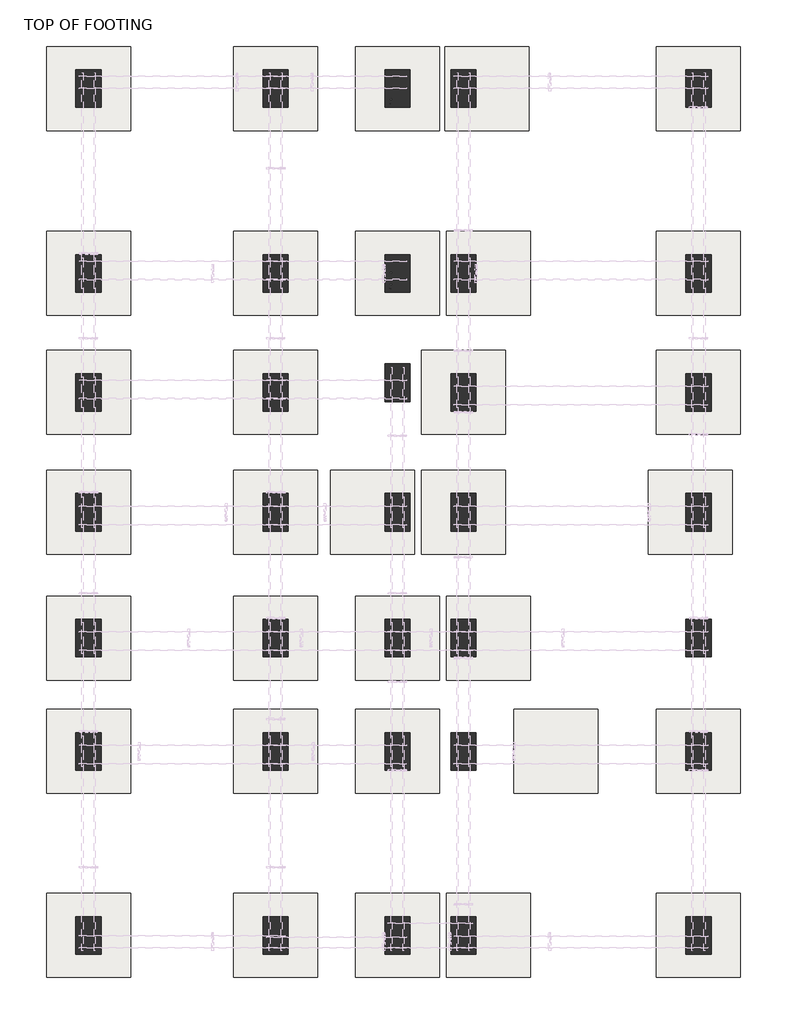
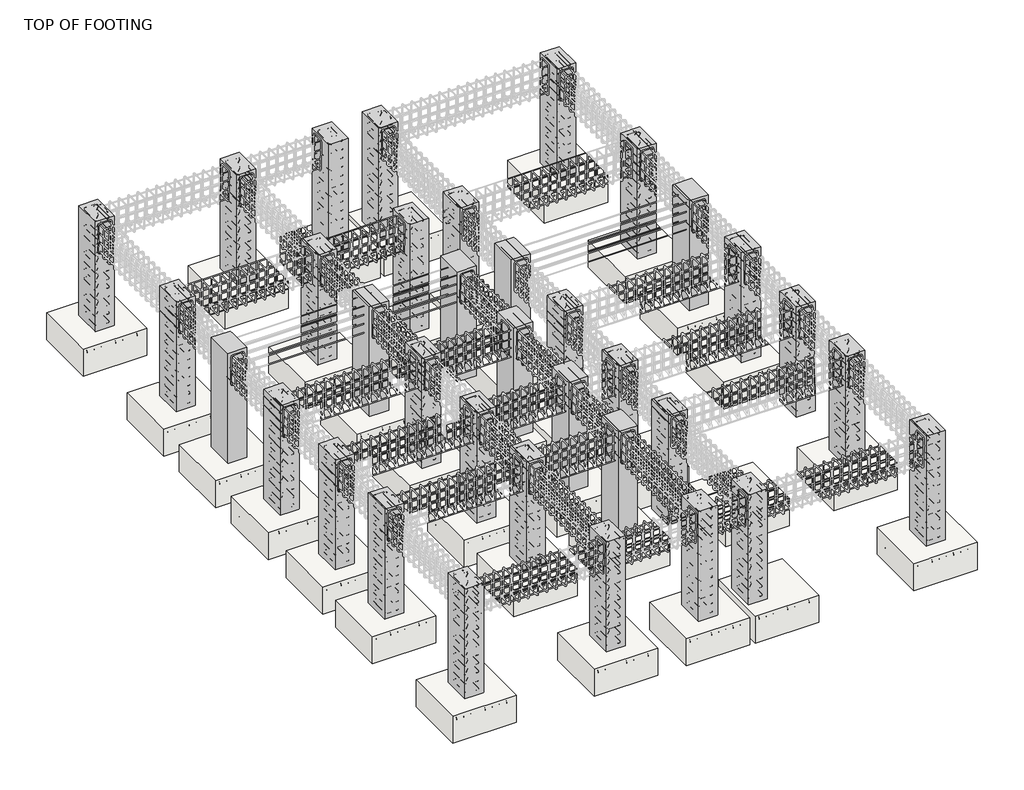
# One storey, part 1 of 19: 35 columns, 33 slabs.
"""IFC4 building model written with IfcOpenShell, lengths in millimetres."""

from ifc_helpers import new_model, si_unit, frame, origin, place, context, project, spatial, polyline, outline, extrude, faceted_brep, transform, mapped, element, save
from components import m_footing_rectangular_4c97ae35

model = new_model("IFC4")

# Units and contexts
model_context = context("Model", 3, world=origin())
ifc_project = project(units=[si_unit("LENGTHUNIT", "METRE", prefix="MILLI")], contexts=[model_context])

# Site, building, storey
site = spatial("IfcSite", under=ifc_project)
building = spatial("IfcBuilding", under=site)
storey = spatial("IfcBuildingStorey", under=building, Name="TOP OF FOOTING", Elevation=-1828.8)

# Columns
placement = place(None, origin())
element("IfcColumn", 1, ObjectType="M_Concrete-Rectangular-Column : 300 x 450mm", at=placement, inside=storey, context=model_context, shape_type="Brep", body=[
    faceted_brep([(-5487.6766954, 9387.4259714, -1828.8), (-5487.6766954, 8937.4259714, -1828.8), (-5787.6766954, 8937.4259714, -1828.8), (-5787.6766954, 9387.4259714, -1828.8), (-5487.6766954, 9387.4259714, 0.0), (-5487.6766954, 9087.4259714, 0.0), (-5487.6766954, 8937.4259714, 0.0), (-5787.6766954, 8937.4259714, 0.0), (-5787.6766954, 9387.4259714, 0.0)], [[[0, 1, 2, 3]], [[4, 5, 6, 1, 0]], [[6, 7, 2, 1]], [[7, 8, 3, 2]], [[8, 4, 0, 3]], [[4, 8, 7, 6, 5]]]),
])
element("IfcColumn", 2, ObjectType="M_Concrete-Rectangular-Column : 300 x 450mm", at=placement, inside=storey, context=model_context, shape_type="Brep", body=[
    faceted_brep([(-3258.2783472, 9387.4259714, -1828.8), (-3258.2783472, 8937.4259714, -1828.8), (-3558.2783472, 8937.4259714, -1828.8), (-3558.2783472, 9387.4259714, -1828.8), (-3258.2783472, 9387.4259714, 0.0), (-3258.2783472, 9087.4259714, 0.0), (-3258.2783472, 8937.4259714, 0.0), (-3558.2783472, 8937.4259714, 0.0), (-3558.2783472, 9087.4259714, 0.0), (-3558.2783472, 9387.4259714, 0.0)], [[[0, 1, 2, 3]], [[4, 5, 6, 1, 0]], [[6, 7, 2, 1]], [[7, 8, 9, 3, 2]], [[9, 4, 0, 3]], [[4, 9, 8, 7, 6, 5]]]),
])
element("IfcColumn", 3, ObjectType="M_Concrete-Rectangular-Column : 300 x 450mm", at=placement, inside=storey, context=model_context, shape_type="Brep", body=[
    faceted_brep([(-1807.6766954, 9387.4259714, -1828.8), (-1807.6766954, 8937.4259714, -1828.8), (-2107.6766954, 8937.4259714, -1828.8), (-2107.6766954, 9387.4259714, -1828.8), (-1807.6766954, 9387.4259714, 0.0), (-1807.6766954, 9087.4259714, 0.0), (-1807.6766954, 8937.4259714, 0.0), (-2107.6766954, 8937.4259714, 0.0), (-2107.6766954, 9087.4259714, 0.0), (-2107.6766954, 9387.4259714, 0.0)], [[[0, 1, 2, 3]], [[4, 5, 6, 1, 0]], [[6, 7, 2, 1]], [[7, 8, 9, 3, 2]], [[9, 4, 0, 3]], [[4, 9, 8, 7, 6, 5]]]),
])
element("IfcColumn", 4, ObjectType="M_Concrete-Rectangular-Column : 300 x 450mm", at=placement, inside=storey, context=model_context, shape_type="Brep", body=[
    faceted_brep([(-1022.4314918, 9387.4259714, -1828.8), (-1022.4314918, 8937.4259714, -1828.8), (-1322.4314918, 8937.4259714, -1828.8), (-1322.4314918, 9387.4259714, -1828.8), (-1022.4314918, 9387.4259714, 0.0), (-1022.4314918, 9087.4259714, 0.0), (-1022.4314918, 8937.4259714, 0.0), (-1322.4314918, 8937.4259714, 0.0), (-1322.4314918, 9087.4259714, 0.0), (-1322.4314918, 9387.4259714, 0.0)], [[[0, 1, 2, 3]], [[4, 5, 6, 1, 0]], [[6, 7, 2, 1]], [[7, 8, 9, 3, 2]], [[9, 4, 0, 3]], [[4, 9, 8, 7, 6, 5]]]),
])
element("IfcColumn", 5, ObjectType="M_Concrete-Rectangular-Column : 300 x 450mm", at=placement, inside=storey, context=model_context, shape_type="Brep", body=[
    faceted_brep([(1777.5685082, 9387.4259714, -1828.8), (1777.5685082, 8937.4259714, -1828.8), (1477.5685082, 8937.4259714, -1828.8), (1477.5685082, 9387.4259714, -1828.8), (1777.5685082, 9387.4259714, 0.0), (1777.5685082, 8937.4259714, 0.0), (1477.5685082, 8937.4259714, 0.0), (1477.5685082, 9087.4259714, 0.0), (1477.5685082, 9387.4259714, 0.0)], [[[0, 1, 2, 3]], [[4, 5, 1, 0]], [[5, 6, 2, 1]], [[6, 7, 8, 3, 2]], [[8, 4, 0, 3]], [[4, 8, 7, 6, 5]]]),
])
element("IfcColumn", 6, ObjectType="M_Concrete-Rectangular-Column : 300 x 450mm", at=placement, inside=storey, context=model_context, shape_type="Brep", body=[
    faceted_brep([(-5487.6766954, 7186.4301143, -1828.8), (-5487.6766954, 6736.4301143, -1828.8), (-5787.6766954, 6736.4301143, -1828.8), (-5787.6766954, 7186.4301143, -1828.8), (-5487.6766954, 7186.4301143, 0.0), (-5487.6766954, 7111.4301143, 0.0), (-5487.6766954, 6811.4301143, 0.0), (-5487.6766954, 6736.4301143, 0.0), (-5787.6766954, 6736.4301143, 0.0), (-5787.6766954, 7186.4301143, 0.0)], [[[0, 1, 2, 3]], [[4, 5, 6, 7, 1, 0]], [[7, 8, 2, 1]], [[8, 9, 3, 2]], [[9, 4, 0, 3]], [[4, 9, 8, 7, 6, 5]]]),
])
element("IfcColumn", 7, ObjectType="M_Concrete-Rectangular-Column : 300 x 450mm", at=placement, inside=storey, context=model_context, shape_type="Brep", body=[
    faceted_brep([(-3258.2783472, 7186.4301143, -1828.8), (-3258.2783472, 6736.4301143, -1828.8), (-3558.2783472, 6736.4301143, -1828.8), (-3558.2783472, 7186.4301143, -1828.8), (-3258.2783472, 7186.4301143, 0.0), (-3258.2783472, 7111.4301143, 0.0), (-3258.2783472, 6811.4301143, 0.0), (-3258.2783472, 6736.4301143, 0.0), (-3258.2783472, 6736.4301143, -300.0), (-3558.2783472, 6736.4301143, 0.0), (-3558.2783472, 6736.4301143, -300.0), (-3558.2783472, 6811.4301143, 0.0), (-3558.2783472, 7111.4301143, 0.0), (-3558.2783472, 7186.4301143, 0.0)], [[[0, 1, 2, 3]], [[1, 0, 4, 5, 6, 7, 8]], [[2, 1, 8, 7, 9, 10]], [[3, 2, 10, 9, 11, 12, 13]], [[0, 3, 13, 4]], [[9, 7, 6, 5, 4, 13, 12, 11]]]),
])
element("IfcColumn", 8, ObjectType="M_Concrete-Rectangular-Column : 300 x 450mm", at=placement, inside=storey, context=model_context, shape_type="Brep", body=[
    faceted_brep([(-1807.6766954, 7186.4301143, -1828.8), (-1807.6766954, 6736.4301143, -1828.8), (-2107.6766954, 6736.4301143, -1828.8), (-2107.6766954, 7186.4301143, -1828.8), (-1807.6766954, 7186.4301143, 0.0), (-1807.6766954, 7111.4301143, 0.0), (-1807.6766954, 6811.4301143, 0.0), (-1807.6766954, 6736.4301143, 0.0), (-1807.6766954, 6736.4301143, -300.0), (-2107.6766954, 6736.4301143, 0.0), (-2107.6766954, 6736.4301143, -300.0), (-2107.6766954, 6811.4301143, 0.0), (-2107.6766954, 7111.4301143, 0.0), (-2107.6766954, 7186.4301143, 0.0)], [[[0, 1, 2, 3]], [[1, 0, 4, 5, 6, 7, 8]], [[2, 1, 8, 7, 9, 10]], [[3, 2, 10, 9, 11, 12, 13]], [[0, 3, 13, 4]], [[9, 7, 6, 5, 4, 13, 12, 11]]]),
])
element("IfcColumn", 9, ObjectType="M_Concrete-Rectangular-Column : 300 x 450mm", at=placement, inside=storey, context=model_context, shape_type="Brep", body=[
    faceted_brep([(-1022.4314918, 7186.4301143, -1828.8), (-1022.4314918, 6736.4301143, -1828.8), (-1322.4314918, 6736.4301143, -1828.8), (-1322.4314918, 7186.4301143, -1828.8), (-1022.4314918, 7186.4301143, 0.0), (-1022.4314918, 7111.4301143, 0.0), (-1022.4314918, 6811.4301143, 0.0), (-1022.4314918, 6736.4301143, 0.0), (-1022.4314918, 6736.4301143, -300.0), (-1322.4314918, 6736.4301143, 0.0), (-1322.4314918, 6736.4301143, -300.0), (-1322.4314918, 6811.4301143, 0.0), (-1322.4314918, 7111.4301143, 0.0), (-1322.4314918, 7186.4301143, 0.0)], [[[0, 1, 2, 3]], [[1, 0, 4, 5, 6, 7, 8]], [[2, 1, 8, 7, 9, 10]], [[3, 2, 10, 9, 11, 12, 13]], [[0, 3, 13, 4]], [[9, 7, 6, 5, 4, 13, 12, 11]]]),
])
element("IfcColumn", 10, ObjectType="M_Concrete-Rectangular-Column : 300 x 450mm", at=placement, inside=storey, context=model_context, shape_type="Brep", body=[
    faceted_brep([(1777.5685082, 7186.4301143, -1828.8), (1777.5685082, 6736.4301143, -1828.8), (1477.5685082, 6736.4301143, -1828.8), (1477.5685082, 7186.4301143, -1828.8), (1777.5685082, 7186.4301143, 0.0), (1777.5685082, 6736.4301143, 0.0), (1477.5685082, 6736.4301143, 0.0), (1477.5685082, 6811.4301143, 0.0), (1477.5685082, 7111.4301143, 0.0), (1477.5685082, 7186.4301143, 0.0)], [[[0, 1, 2, 3]], [[4, 5, 1, 0]], [[5, 6, 2, 1]], [[6, 7, 8, 9, 3, 2]], [[9, 4, 0, 3]], [[4, 9, 8, 7, 6, 5]]]),
])
element("IfcColumn", 11, ObjectType="M_Concrete-Rectangular-Column : 300 x 450mm", at=placement, inside=storey, context=model_context, shape_type="Brep", body=[
    faceted_brep([(-5487.6766954, 5769.9548165, -1828.8), (-5487.6766954, 5319.9548165, -1828.8), (-5787.6766954, 5319.9548165, -1828.8), (-5787.6766954, 5769.9548165, -1828.8), (-5487.6766954, 5769.9548165, 0.0), (-5487.6766954, 5694.9548165, 0.0), (-5487.6766954, 5394.9548165, 0.0), (-5487.6766954, 5319.9548165, 0.0), (-5787.6766954, 5319.9548165, 0.0), (-5787.6766954, 5769.9548165, 0.0)], [[[0, 1, 2, 3]], [[4, 5, 6, 7, 1, 0]], [[7, 8, 2, 1]], [[8, 9, 3, 2]], [[9, 4, 0, 3]], [[4, 9, 8, 7, 6, 5]]]),
])
element("IfcColumn", 12, ObjectType="M_Concrete-Rectangular-Column : 300 x 450mm", at=placement, inside=storey, context=model_context, shape_type="Brep", body=[
    faceted_brep([(-3258.2783472, 5769.9548165, -1828.8), (-3258.2783472, 5319.9548165, -1828.8), (-3558.2783472, 5319.9548165, -1828.8), (-3558.2783472, 5769.9548165, -1828.8), (-3258.2783472, 5769.9548165, -300.0), (-3258.2783472, 5769.9548165, 0.0), (-3258.2783472, 5694.9548165, 0.0), (-3258.2783472, 5394.9548165, 0.0), (-3258.2783472, 5319.9548165, 0.0), (-3258.2783472, 5319.9548165, -300.0), (-3558.2783472, 5319.9548165, 0.0), (-3558.2783472, 5319.9548165, -300.0), (-3558.2783472, 5394.9548165, 0.0), (-3558.2783472, 5694.9548165, 0.0), (-3558.2783472, 5769.9548165, 0.0), (-3558.2783472, 5769.9548165, -300.0)], [[[0, 1, 2, 3]], [[1, 0, 4, 5, 6, 7, 8, 9]], [[2, 1, 9, 8, 10, 11]], [[3, 2, 11, 10, 12, 13, 14, 15]], [[0, 3, 15, 14, 5, 4]], [[10, 8, 7, 6, 5, 14, 13, 12]]]),
])
element("IfcColumn", 13, ObjectType="M_Concrete-Rectangular-Column : 300 x 450mm", at=placement, inside=storey, context=model_context, shape_type="Brep", body=[
    faceted_brep([(-1807.6766954, 5886.4301143, -1828.8), (-1807.6766954, 5436.4301143, -1828.8), (-2107.6766954, 5436.4301143, -1828.8), (-2107.6766954, 5886.4301143, -1828.8), (-1807.6766954, 5886.4301143, -300.0), (-1807.6766954, 5886.4301143, 0.0), (-1807.6766954, 5694.9548165, 0.0), (-1807.6766954, 5436.4301143, 0.0), (-2107.6766954, 5436.4301143, 0.0), (-2107.6766954, 5694.9548165, 0.0), (-2107.6766954, 5886.4301143, 0.0), (-2107.6766954, 5886.4301143, -300.0)], [[[0, 1, 2, 3]], [[1, 0, 4, 5, 6, 7]], [[2, 1, 7, 8]], [[3, 2, 8, 9, 10, 11]], [[0, 3, 11, 10, 5, 4]], [[8, 7, 6, 5, 10, 9]]]),
])
element("IfcColumn", 14, ObjectType="M_Concrete-Rectangular-Column : 300 x 450mm", at=placement, inside=storey, context=model_context, shape_type="Brep", body=[
    faceted_brep([(-1022.4314918, 5769.9548165, -1828.8), (-1022.4314918, 5319.9548165, -1828.8), (-1322.4314918, 5319.9548165, -1828.8), (-1322.4314918, 5769.9548165, -1828.8), (-1022.4314918, 5769.9548165, -300.0), (-1022.4314918, 5769.9548165, 0.0), (-1022.4314918, 5694.9548165, 0.0), (-1022.4314918, 5394.9548165, 0.0), (-1022.4314918, 5319.9548165, 0.0), (-1022.4314918, 5319.9548165, -300.0), (-1322.4314918, 5319.9548165, 0.0), (-1322.4314918, 5319.9548165, -300.0), (-1322.4314918, 5394.9548165, 0.0), (-1322.4314918, 5694.9548165, 0.0), (-1322.4314918, 5769.9548165, 0.0), (-1322.4314918, 5769.9548165, -300.0)], [[[0, 1, 2, 3]], [[1, 0, 4, 5, 6, 7, 8, 9]], [[2, 1, 9, 8, 10, 11]], [[3, 2, 11, 10, 12, 13, 14, 15]], [[0, 3, 15, 14, 5, 4]], [[10, 8, 7, 6, 5, 14, 13, 12]]]),
])
element("IfcColumn", 15, ObjectType="M_Concrete-Rectangular-Column : 300 x 450mm", at=placement, inside=storey, context=model_context, shape_type="Brep", body=[
    faceted_brep([(1777.5685082, 5769.9548165, -1828.8), (1777.5685082, 5319.9548165, -1828.8), (1477.5685082, 5319.9548165, -1828.8), (1477.5685082, 5769.9548165, -1828.8), (1777.5685082, 5769.9548165, 0.0), (1777.5685082, 5319.9548165, 0.0), (1477.5685082, 5319.9548165, 0.0), (1477.5685082, 5394.9548165, 0.0), (1477.5685082, 5694.9548165, 0.0), (1477.5685082, 5769.9548165, 0.0)], [[[0, 1, 2, 3]], [[4, 5, 1, 0]], [[5, 6, 2, 1]], [[6, 7, 8, 9, 3, 2]], [[9, 4, 0, 3]], [[4, 9, 8, 7, 6, 5]]]),
])
element("IfcColumn", 16, ObjectType="M_Concrete-Rectangular-Column : 300 x 450mm", at=placement, inside=storey, context=model_context, shape_type="Brep", body=[
    faceted_brep([(-5487.6766954, 4343.5637574, -1828.8), (-5487.6766954, 3893.5637574, -1828.8), (-5787.6766954, 3893.5637574, -1828.8), (-5787.6766954, 4343.5637574, -1828.8), (-5487.6766954, 4343.5637574, 0.0), (-5487.6766954, 4268.5637574, 0.0), (-5487.6766954, 3968.5637574, 0.0), (-5487.6766954, 3893.5637574, 0.0), (-5787.6766954, 3893.5637574, 0.0), (-5787.6766954, 4343.5637574, 0.0)], [[[0, 1, 2, 3]], [[4, 5, 6, 7, 1, 0]], [[7, 8, 2, 1]], [[8, 9, 3, 2]], [[9, 4, 0, 3]], [[4, 9, 8, 7, 6, 5]]]),
])
element("IfcColumn", 17, ObjectType="M_Concrete-Rectangular-Column : 300 x 450mm", at=placement, inside=storey, context=model_context, shape_type="Brep", body=[
    faceted_brep([(-3258.2783472, 4343.5637574, -1828.8), (-3258.2783472, 3893.5637574, -1828.8), (-3558.2783472, 3893.5637574, -1828.8), (-3558.2783472, 4343.5637574, -1828.8), (-3258.2783472, 4343.5637574, -300.0), (-3258.2783472, 4343.5637574, 0.0), (-3258.2783472, 4268.5637574, 0.0), (-3258.2783472, 3968.5637574, 0.0), (-3258.2783472, 3893.5637574, 0.0), (-3258.2783472, 3893.5637574, -300.0), (-3558.2783472, 3893.5637574, 0.0), (-3558.2783472, 3893.5637574, -300.0), (-3558.2783472, 3968.5637574, 0.0), (-3558.2783472, 4268.5637574, 0.0), (-3558.2783472, 4343.5637574, 0.0), (-3558.2783472, 4343.5637574, -300.0)], [[[0, 1, 2, 3]], [[1, 0, 4, 5, 6, 7, 8, 9]], [[2, 1, 9, 8, 10, 11]], [[3, 2, 11, 10, 12, 13, 14, 15]], [[0, 3, 15, 14, 5, 4]], [[10, 8, 7, 6, 5, 14, 13, 12]]]),
])
element("IfcColumn", 18, ObjectType="M_Concrete-Rectangular-Column : 300 x 450mm", at=placement, inside=storey, context=model_context, shape_type="Brep", body=[
    faceted_brep([(-1807.6766954, 4343.5637574, -1828.8), (-1807.6766954, 3893.5637574, -1828.8), (-2107.6766954, 3893.5637574, -1828.8), (-2107.6766954, 4343.5637574, -1828.8), (-1807.6766954, 4343.5637574, -300.0), (-1807.6766954, 4343.5637574, 0.0), (-1807.6766954, 4268.5637574, 0.0), (-1807.6766954, 3968.5637574, 0.0), (-1807.6766954, 3893.5637574, 0.0), (-1807.6766954, 3893.5637574, -300.0), (-2107.6766954, 3893.5637574, 0.0), (-2107.6766954, 3893.5637574, -300.0), (-2107.6766954, 3968.5637574, 0.0), (-2107.6766954, 4268.5637574, 0.0), (-2107.6766954, 4343.5637574, 0.0), (-2107.6766954, 4343.5637574, -300.0)], [[[0, 1, 2, 3]], [[1, 0, 4, 5, 6, 7, 8, 9]], [[2, 1, 9, 8, 10, 11]], [[3, 2, 11, 10, 12, 13, 14, 15]], [[0, 3, 15, 14, 5, 4]], [[10, 8, 7, 6, 5, 14, 13, 12]]]),
])
element("IfcColumn", 19, ObjectType="M_Concrete-Rectangular-Column : 300 x 450mm", at=placement, inside=storey, context=model_context, shape_type="Brep", body=[
    faceted_brep([(-1022.4314918, 4343.5637574, -1828.8), (-1022.4314918, 3893.5637574, -1828.8), (-1322.4314918, 3893.5637574, -1828.8), (-1322.4314918, 4343.5637574, -1828.8), (-1022.4314918, 4343.5637574, -300.0), (-1022.4314918, 4343.5637574, 0.0), (-1022.4314918, 4268.5637574, 0.0), (-1022.4314918, 3968.5637574, 0.0), (-1022.4314918, 3893.5637574, 0.0), (-1022.4314918, 3893.5637574, -300.0), (-1322.4314918, 3893.5637574, 0.0), (-1322.4314918, 3893.5637574, -300.0), (-1322.4314918, 3968.5637574, 0.0), (-1322.4314918, 4268.5637574, 0.0), (-1322.4314918, 4343.5637574, 0.0), (-1322.4314918, 4343.5637574, -300.0)], [[[0, 1, 2, 3]], [[1, 0, 4, 5, 6, 7, 8, 9]], [[2, 1, 9, 8, 10, 11]], [[3, 2, 11, 10, 12, 13, 14, 15]], [[0, 3, 15, 14, 5, 4]], [[10, 8, 7, 6, 5, 14, 13, 12]]]),
])
element("IfcColumn", 20, ObjectType="M_Concrete-Rectangular-Column : 300 x 450mm", at=placement, inside=storey, context=model_context, shape_type="Brep", body=[
    faceted_brep([(1777.5685082, 4343.5637574, -1828.8), (1777.5685082, 3893.5637574, -1828.8), (1477.5685082, 3893.5637574, -1828.8), (1477.5685082, 4343.5637574, -1828.8), (1777.5685082, 4343.5637574, 0.0), (1777.5685082, 3893.5637574, 0.0), (1477.5685082, 3893.5637574, 0.0), (1477.5685082, 3968.5637574, 0.0), (1477.5685082, 4268.5637574, 0.0), (1477.5685082, 4343.5637574, 0.0)], [[[0, 1, 2, 3]], [[4, 5, 1, 0]], [[5, 6, 2, 1]], [[6, 7, 8, 9, 3, 2]], [[9, 4, 0, 3]], [[4, 9, 8, 7, 6, 5]]]),
])
element("IfcColumn", 21, ObjectType="M_Concrete-Rectangular-Column : 300 x 450mm", at=placement, inside=storey, context=model_context, shape_type="Brep", body=[
    faceted_brep([(-5487.6766954, 2847.1084185, -1828.8), (-5487.6766954, 2397.1084185, -1828.8), (-5787.6766954, 2397.1084185, -1828.8), (-5787.6766954, 2847.1084185, -1828.8), (-5487.6766954, 2847.1084185, 0.0), (-5487.6766954, 2772.1084185, 0.0), (-5487.6766954, 2472.1084185, 0.0), (-5487.6766954, 2397.1084185, 0.0), (-5787.6766954, 2397.1084185, 0.0), (-5787.6766954, 2847.1084185, 0.0)], [[[0, 1, 2, 3]], [[4, 5, 6, 7, 1, 0]], [[7, 8, 2, 1]], [[8, 9, 3, 2]], [[9, 4, 0, 3]], [[4, 9, 8, 7, 6, 5]]]),
])
element("IfcColumn", 22, ObjectType="M_Concrete-Rectangular-Column : 300 x 450mm", at=placement, inside=storey, context=model_context, shape_type="Brep", body=[
    faceted_brep([(-3258.2783472, 2847.1084185, -1828.8), (-3258.2783472, 2397.1084185, -1828.8), (-3558.2783472, 2397.1084185, -1828.8), (-3558.2783472, 2847.1084185, -1828.8), (-3258.2783472, 2847.1084185, -300.0), (-3258.2783472, 2847.1084185, 0.0), (-3258.2783472, 2772.1084185, 0.0), (-3258.2783472, 2472.1084185, 0.0), (-3258.2783472, 2397.1084185, 0.0), (-3258.2783472, 2397.1084185, -300.0), (-3558.2783472, 2397.1084185, 0.0), (-3558.2783472, 2397.1084185, -300.0), (-3558.2783472, 2472.1084185, 0.0), (-3558.2783472, 2772.1084185, 0.0), (-3558.2783472, 2847.1084185, 0.0), (-3558.2783472, 2847.1084185, -300.0)], [[[0, 1, 2, 3]], [[1, 0, 4, 5, 6, 7, 8, 9]], [[2, 1, 9, 8, 10, 11]], [[3, 2, 11, 10, 12, 13, 14, 15]], [[0, 3, 15, 14, 5, 4]], [[10, 8, 7, 6, 5, 14, 13, 12]]]),
])
element("IfcColumn", 23, ObjectType="M_Concrete-Rectangular-Column : 300 x 450mm", at=placement, inside=storey, context=model_context, shape_type="Brep", body=[
    faceted_brep([(-1807.6766954, 2847.1084185, -1828.8), (-1807.6766954, 2397.1084185, -1828.8), (-2107.6766954, 2397.1084185, -1828.8), (-2107.6766954, 2847.1084185, -1828.8), (-1807.6766954, 2847.1084185, -300.0), (-1807.6766954, 2847.1084185, 0.0), (-1807.6766954, 2772.1084185, 0.0), (-1807.6766954, 2472.1084185, 0.0), (-1807.6766954, 2397.1084185, 0.0), (-1807.6766954, 2397.1084185, -300.0), (-2107.6766954, 2397.1084185, 0.0), (-2107.6766954, 2397.1084185, -300.0), (-2107.6766954, 2472.1084185, 0.0), (-2107.6766954, 2772.1084185, 0.0), (-2107.6766954, 2847.1084185, 0.0), (-2107.6766954, 2847.1084185, -300.0)], [[[0, 1, 2, 3]], [[1, 0, 4, 5, 6, 7, 8, 9]], [[2, 1, 9, 8, 10, 11]], [[3, 2, 11, 10, 12, 13, 14, 15]], [[0, 3, 15, 14, 5, 4]], [[10, 8, 7, 6, 5, 14, 13, 12]]]),
])
element("IfcColumn", 24, ObjectType="M_Concrete-Rectangular-Column : 300 x 450mm", at=placement, inside=storey, context=model_context, shape_type="Brep", body=[
    faceted_brep([(-1022.4314918, 2847.1084185, -1828.8), (-1022.4314918, 2397.1084185, -1828.8), (-1322.4314918, 2397.1084185, -1828.8), (-1322.4314918, 2847.1084185, -1828.8), (-1022.4314918, 2847.1084185, -300.0), (-1022.4314918, 2847.1084185, 0.0), (-1022.4314918, 2772.1084185, 0.0), (-1022.4314918, 2472.1084185, 0.0), (-1022.4314918, 2397.1084185, 0.0), (-1022.4314918, 2397.1084185, -300.0), (-1322.4314918, 2397.1084185, 0.0), (-1322.4314918, 2397.1084185, -300.0), (-1322.4314918, 2472.1084185, 0.0), (-1322.4314918, 2772.1084185, 0.0), (-1322.4314918, 2847.1084185, 0.0), (-1322.4314918, 2847.1084185, -300.0)], [[[0, 1, 2, 3]], [[1, 0, 4, 5, 6, 7, 8, 9]], [[2, 1, 9, 8, 10, 11]], [[3, 2, 11, 10, 12, 13, 14, 15]], [[0, 3, 15, 14, 5, 4]], [[10, 8, 7, 6, 5, 14, 13, 12]]]),
])
element("IfcColumn", 25, ObjectType="M_Concrete-Rectangular-Column : 300 x 450mm", at=placement, inside=storey, context=model_context, shape_type="Brep", body=[
    faceted_brep([(1777.5685082, 2847.1084185, -1828.8), (1777.5685082, 2397.1084185, -1828.8), (1477.5685082, 2397.1084185, -1828.8), (1477.5685082, 2847.1084185, -1828.8), (1777.5685082, 2847.1084185, 0.0), (1777.5685082, 2397.1084185, 0.0), (1477.5685082, 2397.1084185, 0.0), (1477.5685082, 2472.1084185, 0.0), (1477.5685082, 2772.1084185, 0.0), (1477.5685082, 2847.1084185, 0.0)], [[[0, 1, 2, 3]], [[4, 5, 1, 0]], [[5, 6, 2, 1]], [[6, 7, 8, 9, 3, 2]], [[9, 4, 0, 3]], [[4, 9, 8, 7, 6, 5]]]),
])
element("IfcColumn", 26, ObjectType="M_Concrete-Rectangular-Column : 300 x 450mm", at=placement, inside=storey, context=model_context, shape_type="Brep", body=[
    faceted_brep([(-5487.6766954, 1496.794883, -1828.8), (-5487.6766954, 1046.794883, -1828.8), (-5787.6766954, 1046.794883, -1828.8), (-5787.6766954, 1496.794883, -1828.8), (-5487.6766954, 1496.794883, 0.0), (-5487.6766954, 1421.794883, 0.0), (-5487.6766954, 1121.794883, 0.0), (-5487.6766954, 1046.794883, 0.0), (-5787.6766954, 1046.794883, 0.0), (-5787.6766954, 1496.794883, 0.0)], [[[0, 1, 2, 3]], [[4, 5, 6, 7, 1, 0]], [[7, 8, 2, 1]], [[8, 9, 3, 2]], [[9, 4, 0, 3]], [[4, 9, 8, 7, 6, 5]]]),
])
element("IfcColumn", 27, ObjectType="M_Concrete-Rectangular-Column : 300 x 450mm", at=placement, inside=storey, context=model_context, shape_type="Brep", body=[
    faceted_brep([(-3258.2783472, 1496.794883, -1828.8), (-3258.2783472, 1046.794883, -1828.8), (-3558.2783472, 1046.794883, -1828.8), (-3558.2783472, 1496.794883, -1828.8), (-3258.2783472, 1496.794883, -300.0), (-3258.2783472, 1496.794883, 0.0), (-3258.2783472, 1421.794883, 0.0), (-3258.2783472, 1121.794883, 0.0), (-3258.2783472, 1046.794883, 0.0), (-3258.2783472, 1046.794883, -300.0), (-3558.2783472, 1046.794883, 0.0), (-3558.2783472, 1046.794883, -300.0), (-3558.2783472, 1121.794883, 0.0), (-3558.2783472, 1421.794883, 0.0), (-3558.2783472, 1496.794883, 0.0), (-3558.2783472, 1496.794883, -300.0)], [[[0, 1, 2, 3]], [[1, 0, 4, 5, 6, 7, 8, 9]], [[2, 1, 9, 8, 10, 11]], [[3, 2, 11, 10, 12, 13, 14, 15]], [[0, 3, 15, 14, 5, 4]], [[10, 8, 7, 6, 5, 14, 13, 12]]]),
])
element("IfcColumn", 28, ObjectType="M_Concrete-Rectangular-Column : 300 x 450mm", at=placement, inside=storey, context=model_context, shape_type="Brep", body=[
    faceted_brep([(-1807.6766954, 1496.794883, -1828.8), (-1807.6766954, 1046.794883, -1828.8), (-2107.6766954, 1046.794883, -1828.8), (-2107.6766954, 1496.794883, -1828.8), (-1807.6766954, 1496.794883, -300.0), (-1807.6766954, 1496.794883, 0.0), (-1807.6766954, 1421.794883, 0.0), (-1807.6766954, 1121.794883, 0.0), (-1807.6766954, 1046.794883, 0.0), (-1807.6766954, 1046.794883, -300.0), (-2107.6766954, 1046.794883, 0.0), (-2107.6766954, 1046.794883, -300.0), (-2107.6766954, 1121.794883, 0.0), (-2107.6766954, 1421.794883, 0.0), (-2107.6766954, 1496.794883, 0.0), (-2107.6766954, 1496.794883, -300.0)], [[[0, 1, 2, 3]], [[1, 0, 4, 5, 6, 7, 8, 9]], [[2, 1, 9, 8, 10, 11]], [[3, 2, 11, 10, 12, 13, 14, 15]], [[0, 3, 15, 14, 5, 4]], [[10, 8, 7, 6, 5, 14, 13, 12]]]),
])
element("IfcColumn", 29, ObjectType="M_Concrete-Rectangular-Column : 300 x 450mm", at=placement, inside=storey, context=model_context, shape_type="Brep", body=[
    faceted_brep([(-1022.4314918, 1496.794883, -1828.8), (-1022.4314918, 1046.794883, -1828.8), (-1322.4314918, 1046.794883, -1828.8), (-1322.4314918, 1496.794883, -1828.8), (-1022.4314918, 1496.794883, -300.0), (-1022.4314918, 1496.794883, 0.0), (-1022.4314918, 1421.794883, 0.0), (-1022.4314918, 1121.794883, 0.0), (-1022.4314918, 1046.794883, 0.0), (-1022.4314918, 1046.794883, -300.0), (-1322.4314918, 1046.794883, 0.0), (-1322.4314918, 1046.794883, -300.0), (-1322.4314918, 1121.794883, 0.0), (-1322.4314918, 1421.794883, 0.0), (-1322.4314918, 1496.794883, 0.0), (-1322.4314918, 1496.794883, -300.0)], [[[0, 1, 2, 3]], [[1, 0, 4, 5, 6, 7, 8, 9]], [[2, 1, 9, 8, 10, 11]], [[3, 2, 11, 10, 12, 13, 14, 15]], [[0, 3, 15, 14, 5, 4]], [[10, 8, 7, 6, 5, 14, 13, 12]]]),
])
element("IfcColumn", 30, ObjectType="M_Concrete-Rectangular-Column : 300 x 450mm", at=placement, inside=storey, context=model_context, shape_type="Brep", body=[
    faceted_brep([(1777.5685082, 1496.794883, -1828.8), (1777.5685082, 1046.794883, -1828.8), (1477.5685082, 1046.794883, -1828.8), (1477.5685082, 1496.794883, -1828.8), (1777.5685082, 1496.794883, 0.0), (1777.5685082, 1046.794883, 0.0), (1477.5685082, 1046.794883, 0.0), (1477.5685082, 1121.794883, 0.0), (1477.5685082, 1421.794883, 0.0), (1477.5685082, 1496.794883, 0.0)], [[[0, 1, 2, 3]], [[4, 5, 1, 0]], [[5, 6, 2, 1]], [[6, 7, 8, 9, 3, 2]], [[9, 4, 0, 3]], [[4, 9, 8, 7, 6, 5]]]),
])
element("IfcColumn", 31, ObjectType="M_Concrete-Rectangular-Column : 300 x 450mm", at=placement, inside=storey, context=model_context, shape_type="Brep", body=[
    faceted_brep([(-5487.6766954, -692.9251006, -1828.8), (-5487.6766954, -1142.9251006, -1828.8), (-5787.6766954, -1142.9251006, -1828.8), (-5787.6766954, -692.9251006, -1828.8), (-5487.6766954, -692.9251006, 0.0), (-5487.6766954, -842.9251006, 0.0), (-5487.6766954, -1142.9251006, 0.0), (-5787.6766954, -1142.9251006, 0.0), (-5787.6766954, -692.9251006, 0.0)], [[[0, 1, 2, 3]], [[4, 5, 6, 1, 0]], [[6, 7, 2, 1]], [[7, 8, 3, 2]], [[8, 4, 0, 3]], [[4, 8, 7, 6, 5]]]),
])
element("IfcColumn", 32, ObjectType="M_Concrete-Rectangular-Column : 300 x 450mm", at=placement, inside=storey, context=model_context, shape_type="Brep", body=[
    faceted_brep([(-3258.2783472, -692.9251006, -1828.8), (-3258.2783472, -1142.9251006, -1828.8), (-3558.2783472, -1142.9251006, -1828.8), (-3558.2783472, -692.9251006, -1828.8), (-3258.2783472, -692.9251006, -300.0), (-3258.2783472, -692.9251006, 0.0), (-3258.2783472, -842.9251006, 0.0), (-3258.2783472, -1142.9251006, 0.0), (-3558.2783472, -1142.9251006, 0.0), (-3558.2783472, -842.9251006, 0.0), (-3558.2783472, -692.9251006, 0.0), (-3558.2783472, -692.9251006, -300.0)], [[[0, 1, 2, 3]], [[1, 0, 4, 5, 6, 7]], [[2, 1, 7, 8]], [[3, 2, 8, 9, 10, 11]], [[0, 3, 11, 10, 5, 4]], [[8, 7, 6, 5, 10, 9]]]),
])
element("IfcColumn", 33, ObjectType="M_Concrete-Rectangular-Column : 300 x 450mm", at=placement, inside=storey, context=model_context, shape_type="Brep", body=[
    faceted_brep([(-1807.6766954, -692.9251006, -1828.8), (-1807.6766954, -1142.9251006, -1828.8), (-2107.6766954, -1142.9251006, -1828.8), (-2107.6766954, -692.9251006, -1828.8), (-1807.6766954, -692.9251006, -300.0), (-1807.6766954, -692.9251006, 0.0), (-1807.6766954, -842.9251006, 0.0), (-1807.6766954, -1142.9251006, 0.0), (-2107.6766954, -1142.9251006, 0.0), (-2107.6766954, -842.9251006, 0.0), (-2107.6766954, -692.9251006, 0.0), (-2107.6766954, -692.9251006, -300.0)], [[[0, 1, 2, 3]], [[1, 0, 4, 5, 6, 7]], [[2, 1, 7, 8]], [[3, 2, 8, 9, 10, 11]], [[0, 3, 11, 10, 5, 4]], [[8, 7, 6, 5, 10, 9]]]),
])
element("IfcColumn", 34, ObjectType="M_Concrete-Rectangular-Column : 300 x 450mm", at=placement, inside=storey, context=model_context, shape_type="Brep", body=[
    faceted_brep([(-1022.4314918, -692.9251006, -1828.8), (-1022.4314918, -1142.9251006, -1828.8), (-1322.4314918, -1142.9251006, -1828.8), (-1322.4314918, -692.9251006, -1828.8), (-1022.4314918, -692.9251006, -300.0), (-1022.4314918, -692.9251006, 0.0), (-1022.4314918, -842.9251006, 0.0), (-1022.4314918, -1142.9251006, 0.0), (-1322.4314918, -1142.9251006, 0.0), (-1322.4314918, -842.9251006, 0.0), (-1322.4314918, -692.9251006, 0.0), (-1322.4314918, -692.9251006, -300.0)], [[[0, 1, 2, 3]], [[1, 0, 4, 5, 6, 7]], [[2, 1, 7, 8]], [[3, 2, 8, 9, 10, 11]], [[0, 3, 11, 10, 5, 4]], [[8, 7, 6, 5, 10, 9]]]),
])
element("IfcColumn", 35, ObjectType="M_Concrete-Rectangular-Column : 300 x 450mm", at=placement, inside=storey, context=model_context, shape_type="Brep", body=[
    faceted_brep([(1777.5685082, -692.9251006, -1828.8), (1777.5685082, -1142.9251006, -1828.8), (1477.5685082, -1142.9251006, -1828.8), (1477.5685082, -692.9251006, -1828.8), (1777.5685082, -692.9251006, 0.0), (1777.5685082, -1142.9251006, 0.0), (1477.5685082, -1142.9251006, 0.0), (1477.5685082, -842.9251006, 0.0), (1477.5685082, -692.9251006, 0.0)], [[[0, 1, 2, 3]], [[4, 5, 1, 0]], [[5, 6, 2, 1]], [[6, 7, 8, 3, 2]], [[8, 4, 0, 3]], [[4, 8, 7, 6, 5]]]),
])

# Slabs
element("IfcSlab", 36, ObjectType="M_Footing-Rectangular", at=placement, inside=storey, context=model_context, shape_type="SweptSolid", body=[
    extrude(outline(polyline([(-1457.6766954, 9662.4259714), (-1457.6766954, 8662.4259714), (-2457.6766954, 8662.4259714), (-2457.6766954, 9662.4259714), (-1457.6766954, 9662.4259714)])), frame((0.0, 0.0, -2278.8), z_axis=(0.0, 0.0, 1.0), x_axis=(1.0, 0.0, 0.0)), (0.0, 0.0, 1.0), 450.0),
])
element("IfcSlab", 37, ObjectType="M_Footing-Rectangular", at=placement, inside=storey, context=model_context, shape_type="SweptSolid", body=[
    extrude(outline(polyline([(-392.4314918, 9662.4259714), (-392.4314918, 8662.4259714), (-1392.4314918, 8662.4259714), (-1392.4314918, 9662.4259714), (-392.4314918, 9662.4259714)])), frame((0.0, 0.0, -2278.8), z_axis=(0.0, 0.0, 1.0), x_axis=(1.0, 0.0, 0.0)), (0.0, 0.0, 1.0), 450.0),
])
m_footing_rectangular_shape = m_footing_rectangular_4c97ae35(model_context)
element("IfcSlab", 38, ObjectType="M_Footing-Rectangular", at=placement, inside=storey, context=model_context, shape_type="MappedRepresentation", body=[
    mapped(m_footing_rectangular_shape, transform((-5637.6766954, 9162.4259714, -1828.8), x_axis=(1.0, 0.0, 0.0), y_axis=(0.0, 1.0, 0.0), z_axis=(0.0, 0.0, 1.0))),
])
element("IfcSlab", 39, ObjectType="M_Footing-Rectangular", at=placement, inside=storey, context=model_context, shape_type="MappedRepresentation", body=[
    mapped(m_footing_rectangular_shape, transform((-3408.2783472, 9162.4259714, -1828.8), x_axis=(1.0, 0.0, 0.0), y_axis=(0.0, 1.0, 0.0), z_axis=(0.0, 0.0, 1.0))),
])
element("IfcSlab", 40, ObjectType="M_Footing-Rectangular", at=placement, inside=storey, context=model_context, shape_type="MappedRepresentation", body=[
    mapped(m_footing_rectangular_shape, transform((1627.5685082, 9162.4259714, -1828.8), x_axis=(1.0, 0.0, 0.0), y_axis=(0.0, 1.0, 0.0), z_axis=(0.0, 0.0, 1.0))),
])
element("IfcSlab", 41, ObjectType="M_Footing-Rectangular", at=placement, inside=storey, context=model_context, shape_type="MappedRepresentation", body=[
    mapped(m_footing_rectangular_shape, transform((-5637.6766954, 6961.4301143, -1828.8), x_axis=(1.0, 0.0, 0.0), y_axis=(0.0, 1.0, 0.0), z_axis=(0.0, 0.0, 1.0))),
])
element("IfcSlab", 42, ObjectType="M_Footing-Rectangular", at=placement, inside=storey, context=model_context, shape_type="MappedRepresentation", body=[
    mapped(m_footing_rectangular_shape, transform((-5637.6766954, 5544.9548165, -1828.8), x_axis=(1.0, 0.0, 0.0), y_axis=(0.0, 1.0, 0.0), z_axis=(0.0, 0.0, 1.0))),
])
element("IfcSlab", 43, ObjectType="M_Footing-Rectangular", at=placement, inside=storey, context=model_context, shape_type="MappedRepresentation", body=[
    mapped(m_footing_rectangular_shape, transform((-3408.2783472, 5544.9548165, -1828.8), x_axis=(1.0, 0.0, 0.0), y_axis=(0.0, 1.0, 0.0), z_axis=(0.0, 0.0, 1.0))),
])
element("IfcSlab", 44, ObjectType="M_Footing-Rectangular", at=placement, inside=storey, context=model_context, shape_type="MappedRepresentation", body=[
    mapped(m_footing_rectangular_shape, transform((-1172.4314918, 5544.9548165, -1828.8), x_axis=(1.0, 0.0, 0.0), y_axis=(0.0, 1.0, 0.0), z_axis=(0.0, 0.0, 1.0))),
])
element("IfcSlab", 45, ObjectType="M_Footing-Rectangular", at=placement, inside=storey, context=model_context, shape_type="MappedRepresentation", body=[
    mapped(m_footing_rectangular_shape, transform((1627.5685082, 5544.9548165, -1828.8), x_axis=(1.0, 0.0, 0.0), y_axis=(0.0, 1.0, 0.0), z_axis=(0.0, 0.0, 1.0))),
])
element("IfcSlab", 46, ObjectType="M_Footing-Rectangular", at=placement, inside=storey, context=model_context, shape_type="MappedRepresentation", body=[
    mapped(m_footing_rectangular_shape, transform((-5637.6766954, -917.9251006, -1828.8), x_axis=(1.0, 0.0, 0.0), y_axis=(0.0, 1.0, 0.0), z_axis=(0.0, 0.0, 1.0))),
])
element("IfcSlab", 47, ObjectType="M_Footing-Rectangular", at=placement, inside=storey, context=model_context, shape_type="MappedRepresentation", body=[
    mapped(m_footing_rectangular_shape, transform((-3408.2783472, -917.9251006, -1828.8), x_axis=(1.0, 0.0, 0.0), y_axis=(0.0, 1.0, 0.0), z_axis=(0.0, 0.0, 1.0))),
])
element("IfcSlab", 48, ObjectType="M_Footing-Rectangular", at=placement, inside=storey, context=model_context, shape_type="MappedRepresentation", body=[
    mapped(m_footing_rectangular_shape, transform((-1957.6766954, -917.9251006, -1828.8), x_axis=(1.0, 0.0, 0.0), y_axis=(0.0, 1.0, 0.0), z_axis=(0.0, 0.0, 1.0))),
])
element("IfcSlab", 49, ObjectType="M_Footing-Rectangular", at=placement, inside=storey, context=model_context, shape_type="MappedRepresentation", body=[
    mapped(m_footing_rectangular_shape, transform((-5637.6766954, 1271.794883, -1828.8), x_axis=(1.0, 0.0, 0.0), y_axis=(0.0, 1.0, 0.0), z_axis=(0.0, 0.0, 1.0))),
])
element("IfcSlab", 50, ObjectType="M_Footing-Rectangular", at=placement, inside=storey, context=model_context, shape_type="MappedRepresentation", body=[
    mapped(m_footing_rectangular_shape, transform((-3408.2783472, 1271.794883, -1828.8), x_axis=(1.0, 0.0, 0.0), y_axis=(0.0, 1.0, 0.0), z_axis=(0.0, 0.0, 1.0))),
])
element("IfcSlab", 51, ObjectType="M_Footing-Rectangular", at=placement, inside=storey, context=model_context, shape_type="MappedRepresentation", body=[
    mapped(m_footing_rectangular_shape, transform((-1957.6766954, 1271.794883, -1828.8), x_axis=(1.0, 0.0, 0.0), y_axis=(0.0, 1.0, 0.0), z_axis=(0.0, 0.0, 1.0))),
])
element("IfcSlab", 52, ObjectType="M_Footing-Rectangular", at=placement, inside=storey, context=model_context, shape_type="MappedRepresentation", body=[
    mapped(m_footing_rectangular_shape, transform((-72.4314918, 1271.794883, -1828.8), x_axis=(1.0, 0.0, 0.0), y_axis=(0.0, 1.0, 0.0), z_axis=(0.0, 0.0, 1.0))),
])
element("IfcSlab", 53, ObjectType="M_Footing-Rectangular", at=placement, inside=storey, context=model_context, shape_type="MappedRepresentation", body=[
    mapped(m_footing_rectangular_shape, transform((1627.5685082, 1271.794883, -1828.8), x_axis=(1.0, 0.0, 0.0), y_axis=(0.0, 1.0, 0.0), z_axis=(0.0, 0.0, 1.0))),
])
element("IfcSlab", 54, ObjectType="M_Footing-Rectangular", at=placement, inside=storey, context=model_context, shape_type="MappedRepresentation", body=[
    mapped(m_footing_rectangular_shape, transform((-5637.6766954, 4118.5637574, -1828.8), x_axis=(1.0, 0.0, 0.0), y_axis=(0.0, 1.0, 0.0), z_axis=(0.0, 0.0, 1.0))),
])
element("IfcSlab", 55, ObjectType="M_Footing-Rectangular", at=placement, inside=storey, context=model_context, shape_type="MappedRepresentation", body=[
    mapped(m_footing_rectangular_shape, transform((1527.5685082, 4118.5637574, -1828.8), x_axis=(1.0, 0.0, 0.0), y_axis=(0.0, 1.0, 0.0), z_axis=(0.0, 0.0, 1.0))),
])
element("IfcSlab", 56, ObjectType="M_Footing-Rectangular", at=placement, inside=storey, context=model_context, shape_type="MappedRepresentation", body=[
    mapped(m_footing_rectangular_shape, transform((-1172.4314918, 4118.5637574, -1828.8), x_axis=(1.0, 0.0, 0.0), y_axis=(0.0, 1.0, 0.0), z_axis=(0.0, 0.0, 1.0))),
])
element("IfcSlab", 57, ObjectType="M_Footing-Rectangular", at=placement, inside=storey, context=model_context, shape_type="MappedRepresentation", body=[
    mapped(m_footing_rectangular_shape, transform((1627.5685082, -917.9251006, -1828.8), x_axis=(1.0, 0.0, 0.0), y_axis=(0.0, 1.0, 0.0), z_axis=(0.0, 0.0, 1.0))),
])
element("IfcSlab", 58, ObjectType="M_Footing-Rectangular", at=placement, inside=storey, context=model_context, shape_type="MappedRepresentation", body=[
    mapped(m_footing_rectangular_shape, transform((-3408.2783472, 6961.4301143, -1828.8), x_axis=(1.0, 0.0, 0.0), y_axis=(0.0, 1.0, 0.0), z_axis=(0.0, 0.0, 1.0))),
])
element("IfcSlab", 59, ObjectType="M_Footing-Rectangular", at=placement, inside=storey, context=model_context, shape_type="MappedRepresentation", body=[
    mapped(m_footing_rectangular_shape, transform((-1957.6766954, 6961.4301143, -1828.8), x_axis=(1.0, 0.0, 0.0), y_axis=(0.0, 1.0, 0.0), z_axis=(0.0, 0.0, 1.0))),
])
element("IfcSlab", 60, ObjectType="M_Footing-Rectangular", at=placement, inside=storey, context=model_context, shape_type="MappedRepresentation", body=[
    mapped(m_footing_rectangular_shape, transform((-872.4314918, 6961.4301143, -1828.8), x_axis=(1.0, 0.0, 0.0), y_axis=(0.0, 1.0, 0.0), z_axis=(0.0, 0.0, 1.0))),
])
element("IfcSlab", 61, ObjectType="M_Footing-Rectangular", at=placement, inside=storey, context=model_context, shape_type="MappedRepresentation", body=[
    mapped(m_footing_rectangular_shape, transform((1627.5685082, 6961.4301143, -1828.8), x_axis=(1.0, 0.0, 0.0), y_axis=(0.0, 1.0, 0.0), z_axis=(0.0, 0.0, 1.0))),
])
element("IfcSlab", 62, ObjectType="M_Footing-Rectangular", at=placement, inside=storey, context=model_context, shape_type="MappedRepresentation", body=[
    mapped(m_footing_rectangular_shape, transform((-3408.2783472, 4118.5637574, -1828.8), x_axis=(1.0, 0.0, 0.0), y_axis=(0.0, 1.0, 0.0), z_axis=(0.0, 0.0, 1.0))),
])
element("IfcSlab", 63, ObjectType="M_Footing-Rectangular", at=placement, inside=storey, context=model_context, shape_type="MappedRepresentation", body=[
    mapped(m_footing_rectangular_shape, transform((-2257.6766954, 4118.5637574, -1828.8), x_axis=(1.0, 0.0, 0.0), y_axis=(0.0, 1.0, 0.0), z_axis=(0.0, 0.0, 1.0))),
])
element("IfcSlab", 64, ObjectType="M_Footing-Rectangular", at=placement, inside=storey, context=model_context, shape_type="MappedRepresentation", body=[
    mapped(m_footing_rectangular_shape, transform((-1957.6766954, 2622.1084185, -1828.8), x_axis=(1.0, 0.0, 0.0), y_axis=(0.0, 1.0, 0.0), z_axis=(0.0, 0.0, 1.0))),
])
element("IfcSlab", 65, ObjectType="M_Footing-Rectangular", at=placement, inside=storey, context=model_context, shape_type="MappedRepresentation", body=[
    mapped(m_footing_rectangular_shape, transform((-872.4314918, 2622.1084185, -1828.8), x_axis=(1.0, 0.0, 0.0), y_axis=(0.0, 1.0, 0.0), z_axis=(0.0, 0.0, 1.0))),
])
element("IfcSlab", 66, ObjectType="M_Footing-Rectangular", at=placement, inside=storey, context=model_context, shape_type="MappedRepresentation", body=[
    mapped(m_footing_rectangular_shape, transform((-3408.2783472, 2622.1084185, -1828.8), x_axis=(1.0, 0.0, 0.0), y_axis=(0.0, 1.0, 0.0), z_axis=(0.0, 0.0, 1.0))),
])
element("IfcSlab", 67, ObjectType="M_Footing-Rectangular", at=placement, inside=storey, context=model_context, shape_type="MappedRepresentation", body=[
    mapped(m_footing_rectangular_shape, transform((-5637.6766954, 2622.1084185, -1828.8), x_axis=(1.0, 0.0, 0.0), y_axis=(0.0, 1.0, 0.0), z_axis=(0.0, 0.0, 1.0))),
])
element("IfcSlab", 68, ObjectType="M_Footing-Rectangular", at=placement, inside=storey, context=model_context, shape_type="MappedRepresentation", body=[
    mapped(m_footing_rectangular_shape, transform((-872.4314918, -917.9251006, -1828.8), x_axis=(1.0, 0.0, 0.0), y_axis=(0.0, 1.0, 0.0), z_axis=(0.0, 0.0, 1.0))),
])

save(model, "model.ifc")

# Revit data of these elements
# Grids (mm)
#   "1": line (3323.28, 9162.426) -> (-6699.816, 9162.426)
#   "2": line (3323.28, 6961.43) -> (-6877.231, 6961.43)
#   "3": line (3323.28, 5544.955) -> (-6877.231, 5544.955)
#   "4": line (3323.28, 4118.564) -> (-6832.024, 4118.564)
#   "5": line (3686.657, 2622.108) -> (-6780.566, 2622.108)
#   "6": line (3686.657, 1271.795) -> (-6877.231, 1271.795)
#   "7": line (3686.657, -917.925) -> (-6877.231, -917.925)
#   "A": line (-5637.677, 9956.957) -> (-5637.677, -2056.742)
#   "B": line (-3408.278, 9956.957) -> (-3408.278, -1939.081)
#   "C": line (-1957.677, 9956.957) -> (-1957.677, -2056.742)
#   "D": line (-1172.431, 9956.957) -> (-1172.431, -2005.523)
#   "E": line (1627.569, 9956.957) -> (1627.569, -2005.523)
# Type "M_Concrete-Rectangular-Column : 300 x 450mm"
#   b = 300 mm
#   h = 450 mm
#   Structural Material [instance default] = Concrete, Cast-in-Place gray
# Type "M_Footing-Rectangular"
#   Width = 1000 mm
#   Length = 1000 mm
#   Foundation Thickness = 450 mm
#   Structural Material [instance default] = Concrete, Cast-in-Place gray
#   Assembly Code = ""
# Elements 1, 2, 3, 4, 5, 6, 7, 8, 9, 10, 11, 12, 13, 14, 15, 16, 17, 18, 19, 20, 21, 22, 23, 24, 25, 26, 27, 28, 29, 30, 31, 32, 33, 34, 35 (IfcColumn, "M_Concrete-Rectangular-Column : 300 x 450mm")
#   Structural Material = Concrete, Cast-in-Place gray
#   Phase Created = New Construction
#   Materials on its faces: "Concrete, Cast-in-Place gray"
# Elements 36, 37, 38, 39, 40, 41, 42, 43, 44, 45, 46, 47, 48, 49, 50, 51, 52, 53, 54, 55, 56, 57, 58, 59, 60, 61, 62, 63, 64, 65, 66, 67, 68 (IfcSlab, "M_Footing-Rectangular")
#   Structural Material = Concrete, Cast-in-Place gray
#   Phase Created = New Construction
#   Materials on its faces: "Concrete, Cast-in-Place gray"
# Materials
#   "Concrete, Cast-in-Place gray": class "Concrete", colour RGB 192 192 192, transparency 0, Description = "Cast-in-place concrete", Cost = 0
